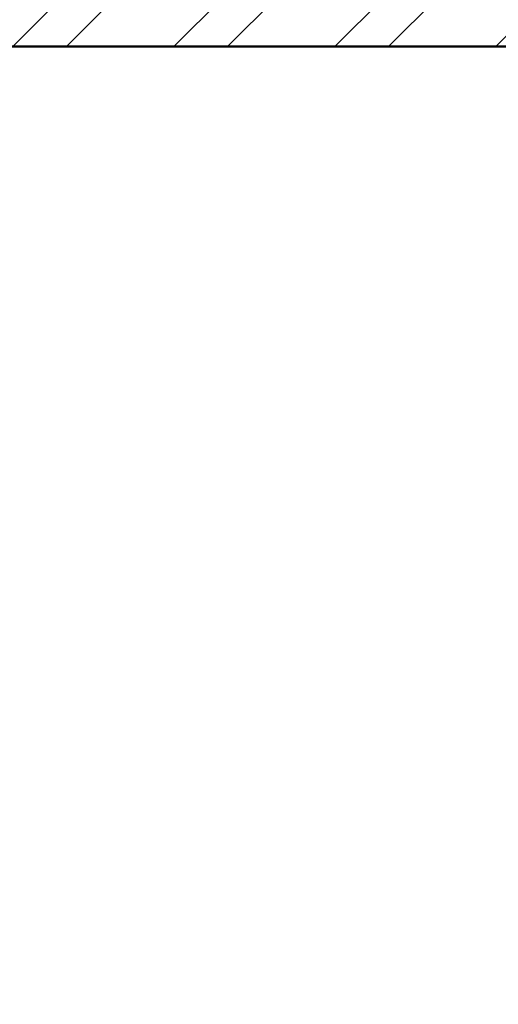
# Model space of a CAD drawing. Units: inches. Extents: x 963 to 2075, y 289 to 2657.
# Tile 86 of 98: x 1556 to 1596, y 2243 to 2325. Entities that reach past the tile are written whole.
import ezdxf

# ---------------------------------------------------------------- set-up
doc = ezdxf.new("R2010")
doc.units = ezdxf.units.IN
doc.layers.add('A-WALL', color=7, linetype='Continuous', lineweight=50)
doc.layers.add('A-WALL-PATT', color=8, linetype='Continuous', lineweight=13)

msp = doc.modelspace()

# ---------------------------------------------------------------- hatches: boundary and pattern name
at = {"layer": 'A-WALL-PATT'}
h = msp.add_hatch(dxfattribs=at)
h.set_pattern_fill('ANSI32', color=256)
h.paths.add_polyline_path([(1296.922, 2558.318), (1203.922, 2558.318), (1203.922, 2493.818), (1191.533, 2493.818), (1191.533, 2489.318), (1211.063, 2489.318), (1211.063, 2492.02), (1211.063, 2493.818), (1208.422, 2493.818), (1208.422, 2553.818), (1292.422, 2553.818), (1292.422, 2538.863), (1296.922, 2538.863)])
h.paths.add_polyline_path([(1442.422, 2558.318), (1349.422, 2558.318), (1349.422, 2538.943), (1353.922, 2538.943), (1353.922, 2553.818), (1437.922, 2553.818), (1437.922, 2493.818), (1434.542, 2493.818), (1434.542, 2489.318), (1448.311, 2489.318), (1448.311, 2491.568), (1448.311, 2493.818), (1442.422, 2493.818)])
h.paths.add_polyline_path([(1415.554, 2491.568), (1415.554, 2493.818), (1340.941, 2493.818), (1340.941, 2489.318), (1371.922, 2489.318), (1371.922, 2378.318), (1367.596, 2378.318), (1367.596, 2373.818), (1371.922, 2373.818), (1371.922, 2355.185), (1376.422, 2355.185), (1376.422, 2489.318), (1415.554, 2489.318)])
h.paths.add_polyline_path([(1304.941, 2491.568), (1304.941, 2493.818), (1296.922, 2493.818), (1296.922, 2514.863), (1292.422, 2514.863), (1292.422, 2493.818), (1232.808, 2493.818), (1232.808, 2489.318), (1256.422, 2489.318), (1256.422, 2327.318), (1253.714, 2327.318), (1253.714, 2322.818), (1328.422, 2322.818), (1328.422, 2331.147), (1323.922, 2331.147), (1323.922, 2327.318), (1260.922, 2327.318), (1260.922, 2373.818), (1323.922, 2373.818), (1323.922, 2357.812), (1328.422, 2357.812), (1328.422, 2373.818), (1346.007, 2373.818), (1346.007, 2376.068), (1346.007, 2378.318), (1260.922, 2378.318), (1260.922, 2489.318), (1304.941, 2489.318)])
h.paths.add_polyline_path([(1226.654, 2327.318), (1124.422, 2327.318), (1124.422, 2347.447), (1119.922, 2347.447), (1119.922, 2322.818), (1163.422, 2322.818), (1163.422, 2305.435), (1165.672, 2305.435), (1167.922, 2305.435), (1167.922, 2322.818), (1226.654, 2322.818), (1226.654, 2325.068)])
h.paths.add_polyline_path([(1095.922, 2489.318), (1124.422, 2489.318), (1131.533, 2489.318), (1131.533, 2491.568), (1131.533, 2493.818), (1119.922, 2493.818), (1091.422, 2493.818), (1091.422, 2417.318), (1095.922, 2417.318), (1119.922, 2417.318), (1119.922, 2407.447), (1124.422, 2407.447), (1124.422, 2421.818), (1095.922, 2421.818)])
h.paths.add_polyline_path([(1512.922, 2558.318), (1508.422, 2558.318), (1508.422, 2493.818), (1503.401, 2493.818), (1503.401, 2489.318), (1508.422, 2489.318), (1508.422, 2327.318), (1376.422, 2327.318), (1376.422, 2330.273), (1371.922, 2330.273), (1371.922, 2298.744), (1376.422, 2298.744), (1376.422, 2322.818), (1508.422, 2322.818), (1508.422, 2165.318), (1504.255, 2165.318), (1504.255, 2160.818), (1508.422, 2160.818), (1508.422, 2108.318), (1512.922, 2108.318), (1512.922, 2160.818), (1516.182, 2160.818), (1516.182, 2163.068), (1516.182, 2165.318), (1512.922, 2165.318), (1512.922, 2322.818), (1644.922, 2322.818), (1644.922, 2298.744), (1649.422, 2298.744), (1649.422, 2322.818), (1649.422, 2330.944), (1647.172, 2330.944), (1644.922, 2330.944), (1644.922, 2327.318), (1512.922, 2327.318), (1512.922, 2489.318), (1516.759, 2489.318), (1516.759, 2491.568), (1516.759, 2493.818), (1512.922, 2493.818)])
h.paths.add_polyline_path([(1671.922, 2558.318), (1578.922, 2558.318), (1578.922, 2493.818), (1573.526, 2493.818), (1573.526, 2489.318), (1586.537, 2489.318), (1586.537, 2491.568), (1586.537, 2493.818), (1583.422, 2493.818), (1583.422, 2553.818), (1667.422, 2553.818), (1667.422, 2541.109), (1671.922, 2541.109)])
h.paths.add_polyline_path([(1681.257, 2493.818), (1671.922, 2493.818), (1671.922, 2517.109), (1667.422, 2517.109), (1667.422, 2493.818), (1610.218, 2493.818), (1610.218, 2489.318), (1644.922, 2489.318), (1644.922, 2357.865), (1649.422, 2357.865), (1649.422, 2373.818), (1652.203, 2373.818), (1652.203, 2375.827), (1652.203, 2378.318), (1649.422, 2378.318), (1649.422, 2489.318), (1681.257, 2489.318), (1681.257, 2491.568)])
h.paths.add_polyline_path([(1821.922, 2558.318), (1728.922, 2558.318), (1728.922, 2541), (1733.422, 2541), (1733.422, 2553.818), (1817.422, 2553.818), (1817.422, 2493.818), (1813.507, 2493.818), (1813.507, 2489.318), (1830.078, 2489.318), (1830.078, 2491.568), (1830.078, 2493.818), (1821.922, 2493.818)])
h.paths.add_polyline_path([(1794.244, 2493.818), (1717.257, 2493.818), (1717.257, 2489.318), (1760.422, 2489.318), (1760.422, 2378.318), (1674.401, 2378.318), (1674.401, 2373.818), (1692.922, 2373.818), (1692.922, 2356.954), (1697.422, 2356.954), (1697.422, 2373.818), (1760.422, 2373.818), (1760.422, 2327.318), (1697.422, 2327.318), (1697.422, 2333.341), (1692.922, 2333.341), (1692.922, 2322.818), (1768.037, 2322.818), (1768.037, 2325.068), (1768.037, 2327.318), (1764.922, 2327.318), (1764.922, 2489.318), (1794.244, 2489.318)])
h.paths.add_polyline_path([(1733.422, 2517), (1728.922, 2517), (1728.922, 2493.818), (1733.422, 2493.818)], flags=17)
h.paths.add_polyline_path([(1929.922, 2493.818), (1890.078, 2493.818), (1890.078, 2489.318), (1896.922, 2489.318), (1925.422, 2489.318), (1925.422, 2421.818), (1896.922, 2421.818), (1896.922, 2408.318), (1901.422, 2408.318), (1901.422, 2417.318), (1925.422, 2417.318), (1929.922, 2417.318)])
h.paths.add_polyline_path([(1901.422, 2348.318), (1896.922, 2348.318), (1896.922, 2327.318), (1800.423, 2327.318), (1800.423, 2322.818), (1853.422, 2322.818), (1853.422, 2309.453), (1857.922, 2309.453), (1857.922, 2322.818), (1901.422, 2322.818)])
h.paths.add_polyline_path([(1857.922, 2249.453), (1853.422, 2249.453), (1853.422, 2214.818), (1686.309, 2214.818), (1686.309, 2210.318), (1853.422, 2210.318), (1853.422, 2202.134), (1857.922, 2202.134), (1857.922, 2210.318)])
h.paths.add_polyline_path([(1857.922, 2142.134), (1853.422, 2142.134), (1853.422, 2115.422), (1841.422, 2115.422), (1841.422, 2088.531), (1841.422, 2046.949), (1845.922, 2046.949), (1845.922, 2110.922), (1905.922, 2110.922), (1905.922, 2092.517), (1910.422, 2092.517), (1910.422, 2115.422), (1857.922, 2115.422)])
h.paths.add_polyline_path([(1532.436, 1482.342), (1573.456, 1482.342), (1573.456, 1501), (1532.436, 1501)], flags=9)
h.paths.add_polyline_path([(1438.658, 1486.302), (1479.678, 1486.302), (1479.678, 1504.96), (1438.658, 1504.96)], flags=9)
h.paths.add_polyline_path([(1411.215, 1365.308), (1659.139, 1365.308), (1659.139, 1402.401), (1411.215, 1402.401)], flags=9)
h.paths.add_polyline_path([(1185.671, 2296.298), (1248.16, 2296.298), (1248.16, 2314.955), (1185.671, 2314.955)], flags=9)
h.paths.add_polyline_path([(1177.31, 2187.35), (1216.15, 2187.35), (1216.15, 2206.007), (1177.31, 2206.007)], flags=9)
h.paths.add_polyline_path([(1295.101, 1602.083), (1328.26, 1602.083), (1328.26, 1620.741), (1295.101, 1620.741)], flags=9)
h.paths.add_polyline_path([(1525.126, 2005.99), (1558.39, 2005.99), (1558.39, 2024.648), (1525.126, 2024.648)], flags=9)
h.paths.add_polyline_path([(1459.606, 1977.125), (1472.195, 1977.125), (1472.195, 1987.429), (1459.606, 1987.429)], flags=9)
h.paths.add_polyline_path([(1467.815, 2053.676), (1480.018, 2053.676), (1480.018, 2063.979), (1467.815, 2063.979)], flags=9)
h.paths.add_polyline_path([(1555.184, 2119.02), (1584.563, 2119.02), (1584.563, 2137.678), (1555.184, 2137.678)], flags=25)
h.paths.add_polyline_path([(1405.389, 2115.291), (1444.478, 2115.291), (1444.478, 2133.948), (1405.389, 2133.948)], flags=25)
h.paths.add_polyline_path([(1698.482, 2004.259), (1727.695, 2004.259), (1727.695, 2022.916), (1698.482, 2022.916)], flags=9)
h.paths.add_polyline_path([(1612.158, 1972.855), (1629.016, 1972.855), (1629.016, 1983.159), (1612.158, 1983.159)], flags=9)
h.paths.add_polyline_path([(1608.289, 2060.036), (1625.147, 2060.036), (1625.147, 2070.34), (1608.289, 2070.34)], flags=9)
h.paths.add_polyline_path([(1527.954, 1684.402), (1566.795, 1684.402), (1566.795, 1703.06), (1527.954, 1703.06)], flags=9)
h.paths.add_polyline_path([(1422.792, 1683.59), (1461.633, 1683.59), (1461.633, 1702.247), (1422.792, 1702.247)], flags=9)
h.paths.add_polyline_path([(1531.262, 1732.459), (1574.015, 1732.459), (1574.015, 1751.116), (1531.262, 1751.116)], flags=9)
h.paths.add_polyline_path([(1402.872, 1732.845), (1439.799, 1732.845), (1439.799, 1751.502), (1402.872, 1751.502)], flags=9)
h.paths.add_polyline_path([(1243.122, 1923.132), (1281.962, 1923.132), (1281.962, 1941.79), (1243.122, 1941.79)], flags=9)
h.paths.add_polyline_path([(1181.752, 1792.268), (1244.241, 1792.268), (1244.241, 1810.926), (1181.752, 1810.926)], flags=9)
h.paths.add_polyline_path([(1265.822, 1670.3), (1316.071, 1670.3), (1316.071, 1688.957), (1265.822, 1688.957)], flags=9)
h.paths.add_polyline_path([(1140.263, 1676.054), (1179.104, 1676.054), (1179.104, 1694.711), (1140.263, 1694.711)], flags=9)
h.paths.add_polyline_path([(1107.49, 1490.889), (1143.374, 1490.889), (1143.374, 1509.546), (1107.49, 1509.546)], flags=9)
h.paths.add_polyline_path([(1217.584, 1483.899), (1246.741, 1483.899), (1246.741, 1502.556), (1217.584, 1502.556)], flags=9)
h.paths.add_polyline_path([(1389.21, 1486.919), (1418.367, 1486.919), (1418.367, 1505.576), (1389.21, 1505.576)], flags=9)
h.paths.add_polyline_path([(1672.208, 1602.083), (1705.366, 1602.083), (1705.366, 1620.741), (1672.208, 1620.741)], flags=9)
h.paths.add_polyline_path([(1752.082, 1522.638), (1781.24, 1522.638), (1781.24, 1541.295), (1752.082, 1541.295)], flags=9)
h.paths.add_polyline_path([(1848.275, 1491.26), (1884.158, 1491.26), (1884.158, 1509.918), (1848.275, 1509.918)], flags=9)
h.paths.add_polyline_path([(1822.47, 1685.62), (1861.31, 1685.62), (1861.31, 1704.278), (1822.47, 1704.278)], flags=9)
h.paths.add_polyline_path([(1713.195, 1672.232), (1763.444, 1672.232), (1763.444, 1690.889), (1713.195, 1690.889)], flags=9)
h.paths.add_polyline_path([(1736.619, 1790.578), (1799.109, 1790.578), (1799.109, 1809.235), (1736.619, 1809.235)], flags=9)
h.paths.add_polyline_path([(1691.491, 1916.355), (1730.332, 1916.355), (1730.332, 1935.013), (1691.491, 1935.013)], flags=9)
h.paths.add_polyline_path([(1764.872, 1973.922), (1794.306, 1973.922), (1794.306, 1992.58), (1764.872, 1992.58)], flags=9)
h.paths.add_polyline_path([(1767.854, 2034.017), (1797.288, 2034.017), (1797.288, 2052.674), (1767.854, 2052.674)], flags=9)
h.paths.add_polyline_path([(1851.593, 2060.331), (1880.751, 2060.331), (1880.751, 2078.989), (1851.593, 2078.989)], flags=25)
h.paths.add_polyline_path([(1688.491, 2086.874), (1727.332, 2086.874), (1727.332, 2105.531), (1688.491, 2105.531)], flags=9)
h.paths.add_polyline_path([(1537.743, 2293.581), (1580.495, 2293.581), (1580.495, 2312.239), (1537.743, 2312.239)], flags=25)
h.paths.add_polyline_path([(1425.587, 2296.109), (1468.34, 2296.109), (1468.34, 2314.766), (1425.587, 2314.766)], flags=25)
h.paths.add_polyline_path([(1278.518, 2004.184), (1307.72, 2004.184), (1307.72, 2022.841), (1278.518, 2022.841)], flags=9)
h.paths.add_polyline_path([(1193.282, 1973.635), (1222.715, 1973.635), (1222.715, 1992.292), (1193.282, 1992.292)], flags=9)
h.paths.add_polyline_path([(1192.411, 2040.577), (1221.845, 2040.577), (1221.845, 2059.234), (1192.411, 2059.234)], flags=9)
h.paths.add_polyline_path([(1130.603, 1951.393), (1159.76, 1951.393), (1159.76, 1970.05), (1130.603, 1970.05)], flags=9)
h.paths.add_polyline_path([(1132.827, 2052.494), (1161.984, 2052.494), (1161.984, 2071.151), (1132.827, 2071.151)], flags=9)
h.paths.add_polyline_path([(1265.128, 2334.619), (1315.377, 2334.619), (1315.377, 2353.277), (1265.128, 2353.277)], flags=25)
h.paths.add_polyline_path([(1136.741, 2330.785), (1175.582, 2330.785), (1175.582, 2349.443), (1136.741, 2349.443)], flags=9)
h.paths.add_polyline_path([(1287.422, 2417.204), (1320.58, 2417.204), (1320.58, 2435.861), (1287.422, 2435.861)], flags=25)
h.paths.add_polyline_path([(1430.988, 2329.159), (1469.828, 2329.159), (1469.828, 2347.816), (1430.988, 2347.816)], flags=25)
h.paths.add_polyline_path([(1525.424, 2329.213), (1564.264, 2329.213), (1564.264, 2347.87), (1525.424, 2347.87)], flags=25)
h.paths.add_polyline_path([(1684.525, 2382.799), (1717.683, 2382.799), (1717.683, 2401.457), (1684.525, 2401.457)], flags=25)
h.paths.add_polyline_path([(1704.805, 2340.293), (1755.054, 2340.293), (1755.054, 2358.95), (1704.805, 2358.95)], flags=25)
h.paths.add_polyline_path([(1694.113, 2287.757), (1756.602, 2287.757), (1756.602, 2306.414), (1694.113, 2306.414)], flags=9)
h.paths.add_polyline_path([(1815.778, 2329.861), (1854.618, 2329.861), (1854.618, 2348.518), (1815.778, 2348.518)], flags=9)
h.paths.add_polyline_path([(1842.873, 2514.256), (1878.756, 2514.256), (1878.756, 2532.914), (1842.873, 2532.914)], flags=9)
h.paths.add_polyline_path([(1769.513, 2531.447), (1798.671, 2531.447), (1798.671, 2550.104), (1769.513, 2550.104)], flags=25)
h.paths.add_polyline_path([(1594.772, 2518.468), (1623.93, 2518.468), (1623.93, 2537.125), (1594.772, 2537.125)], flags=25)
h.paths.add_polyline_path([(1520.723, 2516.185), (1556.606, 2516.185), (1556.606, 2534.842), (1520.723, 2534.842)], flags=25)
h.paths.add_polyline_path([(1464.456, 2516.694), (1500.34, 2516.694), (1500.34, 2535.351), (1464.456, 2535.351)], flags=25)
h.paths.add_polyline_path([(1365.696, 2528.97), (1394.854, 2528.97), (1394.854, 2547.627), (1365.696, 2547.627)], flags=25)
h.paths.add_polyline_path([(1222.838, 2516.231), (1251.995, 2516.231), (1251.995, 2534.889), (1222.838, 2534.889)], flags=25)
h.paths.add_polyline_path([(1104.545, 2509.6), (1140.429, 2509.6), (1140.429, 2528.257), (1104.545, 2528.257)], flags=9)
h = msp.add_hatch(dxfattribs=at)
h.set_pattern_fill('ANSI32', color=256)
h.paths.add_polyline_path([(1335.968, 2212.568), (1335.968, 2214.818), (1167.922, 2214.818), (1167.922, 2245.435), (1163.422, 2245.435), (1163.422, 2210.318), (1163.422, 2194.812), (1167.922, 2194.812), (1167.922, 2210.318), (1335.968, 2210.318)])
h.paths.add_polyline_path([(1532.436, 1482.342), (1573.456, 1482.342), (1573.456, 1501), (1532.436, 1501)], flags=9)
h.paths.add_polyline_path([(1438.658, 1486.302), (1479.678, 1486.302), (1479.678, 1504.96), (1438.658, 1504.96)], flags=9)
h.paths.add_polyline_path([(1411.215, 1365.308), (1659.139, 1365.308), (1659.139, 1402.401), (1411.215, 1402.401)], flags=9)
h.paths.add_polyline_path([(1185.671, 2296.298), (1248.16, 2296.298), (1248.16, 2314.955), (1185.671, 2314.955)], flags=9)
h.paths.add_polyline_path([(1177.31, 2187.35), (1216.15, 2187.35), (1216.15, 2206.007), (1177.31, 2206.007)], flags=9)
h.paths.add_polyline_path([(1295.101, 1602.083), (1328.26, 1602.083), (1328.26, 1620.741), (1295.101, 1620.741)], flags=9)
h.paths.add_polyline_path([(1525.126, 2005.99), (1558.39, 2005.99), (1558.39, 2024.648), (1525.126, 2024.648)], flags=9)
h.paths.add_polyline_path([(1459.606, 1977.125), (1472.195, 1977.125), (1472.195, 1987.429), (1459.606, 1987.429)], flags=9)
h.paths.add_polyline_path([(1467.815, 2053.676), (1480.018, 2053.676), (1480.018, 2063.979), (1467.815, 2063.979)], flags=9)
h.paths.add_polyline_path([(1555.184, 2119.02), (1584.563, 2119.02), (1584.563, 2137.678), (1555.184, 2137.678)], flags=9)
h.paths.add_polyline_path([(1405.389, 2115.291), (1444.478, 2115.291), (1444.478, 2133.948), (1405.389, 2133.948)], flags=9)
h.paths.add_polyline_path([(1698.482, 2004.259), (1727.695, 2004.259), (1727.695, 2022.916), (1698.482, 2022.916)], flags=9)
h.paths.add_polyline_path([(1612.158, 1972.855), (1629.016, 1972.855), (1629.016, 1983.159), (1612.158, 1983.159)], flags=9)
h.paths.add_polyline_path([(1608.289, 2060.036), (1625.147, 2060.036), (1625.147, 2070.34), (1608.289, 2070.34)], flags=9)
h.paths.add_polyline_path([(1527.954, 1684.402), (1566.795, 1684.402), (1566.795, 1703.06), (1527.954, 1703.06)], flags=9)
h.paths.add_polyline_path([(1422.792, 1683.59), (1461.633, 1683.59), (1461.633, 1702.247), (1422.792, 1702.247)], flags=9)
h.paths.add_polyline_path([(1531.262, 1732.459), (1574.015, 1732.459), (1574.015, 1751.116), (1531.262, 1751.116)], flags=9)
h.paths.add_polyline_path([(1402.872, 1732.845), (1439.799, 1732.845), (1439.799, 1751.502), (1402.872, 1751.502)], flags=9)
h.paths.add_polyline_path([(1243.122, 1923.132), (1281.962, 1923.132), (1281.962, 1941.79), (1243.122, 1941.79)], flags=9)
h.paths.add_polyline_path([(1181.752, 1792.268), (1244.241, 1792.268), (1244.241, 1810.926), (1181.752, 1810.926)], flags=9)
h.paths.add_polyline_path([(1265.822, 1670.3), (1316.071, 1670.3), (1316.071, 1688.957), (1265.822, 1688.957)], flags=9)
h.paths.add_polyline_path([(1140.263, 1676.054), (1179.104, 1676.054), (1179.104, 1694.711), (1140.263, 1694.711)], flags=9)
h.paths.add_polyline_path([(1107.49, 1490.889), (1143.374, 1490.889), (1143.374, 1509.546), (1107.49, 1509.546)], flags=9)
h.paths.add_polyline_path([(1217.584, 1483.899), (1246.741, 1483.899), (1246.741, 1502.556), (1217.584, 1502.556)], flags=9)
h.paths.add_polyline_path([(1389.21, 1486.919), (1418.367, 1486.919), (1418.367, 1505.576), (1389.21, 1505.576)], flags=9)
h.paths.add_polyline_path([(1672.208, 1602.083), (1705.366, 1602.083), (1705.366, 1620.741), (1672.208, 1620.741)], flags=9)
h.paths.add_polyline_path([(1752.082, 1522.638), (1781.24, 1522.638), (1781.24, 1541.295), (1752.082, 1541.295)], flags=9)
h.paths.add_polyline_path([(1848.275, 1491.26), (1884.158, 1491.26), (1884.158, 1509.918), (1848.275, 1509.918)], flags=9)
h.paths.add_polyline_path([(1822.47, 1685.62), (1861.31, 1685.62), (1861.31, 1704.278), (1822.47, 1704.278)], flags=9)
h.paths.add_polyline_path([(1713.195, 1672.232), (1763.444, 1672.232), (1763.444, 1690.889), (1713.195, 1690.889)], flags=9)
h.paths.add_polyline_path([(1736.619, 1790.578), (1799.109, 1790.578), (1799.109, 1809.235), (1736.619, 1809.235)], flags=9)
h.paths.add_polyline_path([(1691.491, 1916.355), (1730.332, 1916.355), (1730.332, 1935.013), (1691.491, 1935.013)], flags=9)
h.paths.add_polyline_path([(1764.872, 1973.922), (1794.306, 1973.922), (1794.306, 1992.58), (1764.872, 1992.58)], flags=9)
h.paths.add_polyline_path([(1767.854, 2034.017), (1797.288, 2034.017), (1797.288, 2052.674), (1767.854, 2052.674)], flags=9)
h.paths.add_polyline_path([(1851.593, 2060.331), (1880.751, 2060.331), (1880.751, 2078.989), (1851.593, 2078.989)], flags=9)
h.paths.add_polyline_path([(1688.491, 2086.874), (1727.332, 2086.874), (1727.332, 2105.531), (1688.491, 2105.531)], flags=9)
h.paths.add_polyline_path([(1537.743, 2293.581), (1580.495, 2293.581), (1580.495, 2312.239), (1537.743, 2312.239)], flags=9)
h.paths.add_polyline_path([(1425.587, 2296.109), (1468.34, 2296.109), (1468.34, 2314.766), (1425.587, 2314.766)], flags=9)
h.paths.add_polyline_path([(1278.518, 2004.184), (1307.72, 2004.184), (1307.72, 2022.841), (1278.518, 2022.841)], flags=9)
h.paths.add_polyline_path([(1193.282, 1973.635), (1222.715, 1973.635), (1222.715, 1992.292), (1193.282, 1992.292)], flags=9)
h.paths.add_polyline_path([(1192.411, 2040.577), (1221.845, 2040.577), (1221.845, 2059.234), (1192.411, 2059.234)], flags=9)
h.paths.add_polyline_path([(1130.603, 1951.393), (1159.76, 1951.393), (1159.76, 1970.05), (1130.603, 1970.05)], flags=9)
h.paths.add_polyline_path([(1132.827, 2052.494), (1161.984, 2052.494), (1161.984, 2071.151), (1132.827, 2071.151)], flags=9)
h.paths.add_polyline_path([(1265.128, 2334.619), (1315.377, 2334.619), (1315.377, 2353.277), (1265.128, 2353.277)], flags=9)
h.paths.add_polyline_path([(1136.741, 2330.785), (1175.582, 2330.785), (1175.582, 2349.443), (1136.741, 2349.443)], flags=9)
h.paths.add_polyline_path([(1287.422, 2417.204), (1320.58, 2417.204), (1320.58, 2435.861), (1287.422, 2435.861)], flags=9)
h.paths.add_polyline_path([(1430.988, 2329.159), (1469.828, 2329.159), (1469.828, 2347.816), (1430.988, 2347.816)], flags=9)
h.paths.add_polyline_path([(1525.424, 2329.213), (1564.264, 2329.213), (1564.264, 2347.87), (1525.424, 2347.87)], flags=9)
h.paths.add_polyline_path([(1684.525, 2382.799), (1717.683, 2382.799), (1717.683, 2401.457), (1684.525, 2401.457)], flags=9)
h.paths.add_polyline_path([(1704.805, 2340.293), (1755.054, 2340.293), (1755.054, 2358.95), (1704.805, 2358.95)], flags=9)
h.paths.add_polyline_path([(1694.113, 2287.757), (1756.602, 2287.757), (1756.602, 2306.414), (1694.113, 2306.414)], flags=9)
h.paths.add_polyline_path([(1815.778, 2329.861), (1854.618, 2329.861), (1854.618, 2348.518), (1815.778, 2348.518)], flags=9)
h.paths.add_polyline_path([(1842.873, 2514.256), (1878.756, 2514.256), (1878.756, 2532.914), (1842.873, 2532.914)], flags=9)
h.paths.add_polyline_path([(1769.513, 2531.447), (1798.671, 2531.447), (1798.671, 2550.104), (1769.513, 2550.104)], flags=9)
h.paths.add_polyline_path([(1594.772, 2518.468), (1623.93, 2518.468), (1623.93, 2537.125), (1594.772, 2537.125)], flags=9)
h.paths.add_polyline_path([(1520.723, 2516.185), (1556.606, 2516.185), (1556.606, 2534.842), (1520.723, 2534.842)], flags=9)
h.paths.add_polyline_path([(1464.456, 2516.694), (1500.34, 2516.694), (1500.34, 2535.351), (1464.456, 2535.351)], flags=9)
h.paths.add_polyline_path([(1365.696, 2528.97), (1394.854, 2528.97), (1394.854, 2547.627), (1365.696, 2547.627)], flags=9)
h.paths.add_polyline_path([(1222.838, 2516.231), (1251.995, 2516.231), (1251.995, 2534.889), (1222.838, 2534.889)], flags=9)
h.paths.add_polyline_path([(1104.545, 2509.6), (1140.429, 2509.6), (1140.429, 2528.257), (1104.545, 2528.257)], flags=9)

# ---------------------------------------------------------------- linework, layer by layer
at = {"layer": 'A-WALL'}
msp.add_line((1512.922, 2322.818), (1644.922, 2322.818), dxfattribs=at)

doc.saveas('drawing.dxf')
